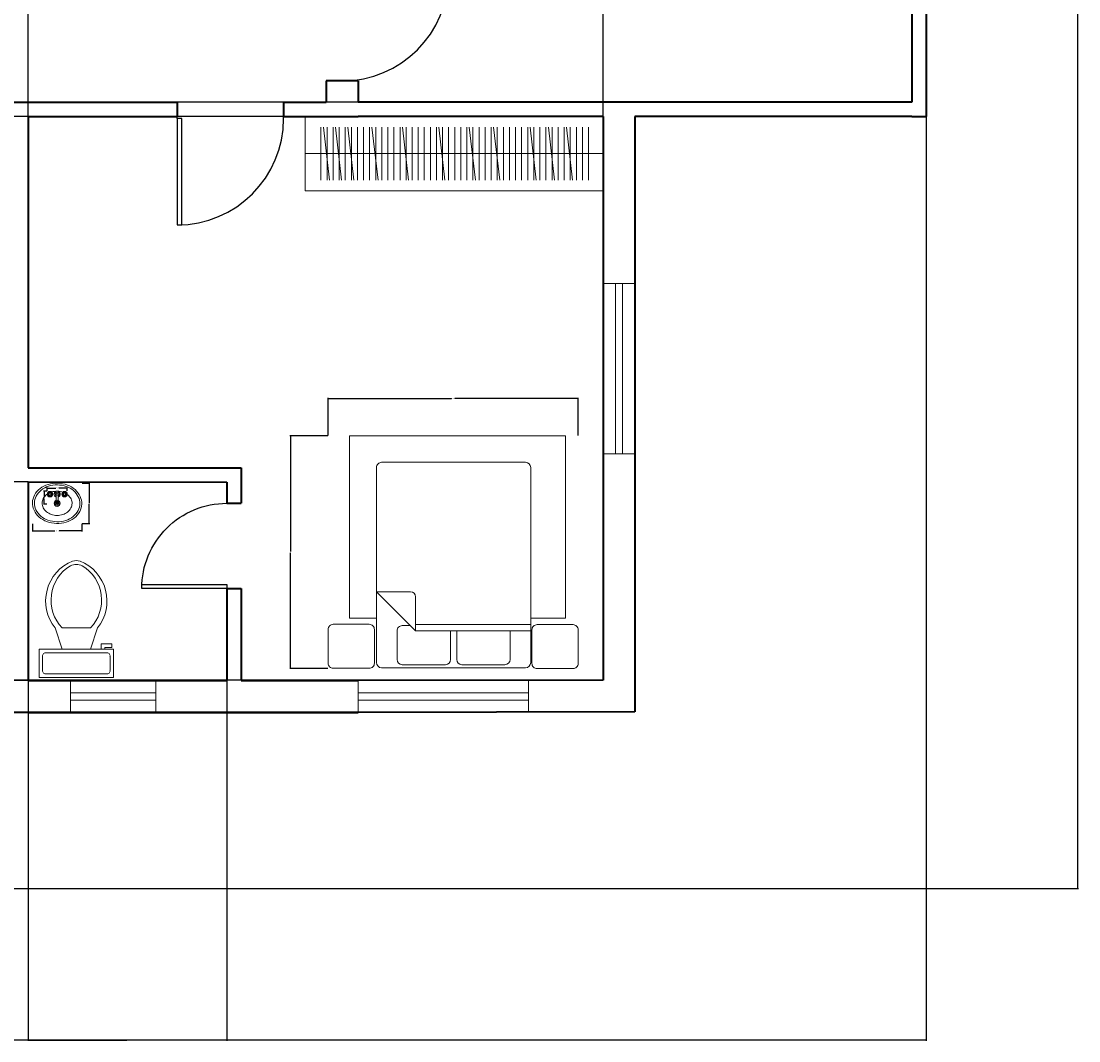
# Model space of a CAD drawing. Units: inches. Extents: x 2024 to 2965, y 1692 to 2308.
# Tile 5 of 8: x 2667 to 2965, y 1692 to 1980. Entities that reach past the tile are written whole.
import ezdxf

# ---------------------------------------------------------------- set-up
doc = ezdxf.new("R2010")
doc.units = ezdxf.units.IN
for name, color, linetype, lineweight in [('A-ANNO-DIMS', 2, 'Continuous', 18), ('A-DOOR', 3, 'Continuous', 25), ('A-FLOR-CASE', 33, 'Continuous', 20), ('A-FLOR-CASE-PATT', 252, 'Continuous', 13), ('A-FLOR-FIXT', 9, 'Continuous', 18), ('A-FURN', 8, 'Continuous', 18), ('A-GLAZ', 4, 'Continuous', 18), ('A-WALL', 7, 'Continuous', 35)]:
    doc.layers.add(name, color=color, linetype=linetype, lineweight=lineweight)
doc.styles.get("Standard").update_dxf_attribs({"font": 'arial.ttf'})
doc.dimstyles.get("Standard").update_dxf_attribs({"dimtxt": 0.18, "dimasz": 0.18, "dimexe": 0.18, "dimexo": 0.0625, "dimgap": 0.09, "dimtad": 0, "dimtih": 1, "dimtoh": 1, "dimdec": 4, "dimzin": 0, "dimdsep": 46, "dimtxsty": 'Standard', "dimcen": 0.09, "dimadec": 0, "dimazin": 0, "dimtfac": 1, "dimtdec": 4, "dimtofl": 0, "dimtmove": 0, "dimatfit": 3, "dimfxl": 1, "dimtolj": 1, "dimtzin": 0, "dimarcsym": 0})

# ---------------------------------------------------------------- blocks, each defined once
blk = doc.blocks.new('*U6')
for p, q in [((0, 0), (0, 6)), ((40, 0), (40, 6))]:
    blk.add_line(p, q)
blk.add_lwpolyline([(0, 0), (0, -40), (1.75, -40), (1.75, 0)], close=True)
blk.add_arc((0, 0), 40, 270, 0)
blk = doc.blocks.new('*U7')
for p, q in [((0, 0), (0, -6)), ((40, 0), (40, -6))]:
    blk.add_line(p, q)
blk.add_lwpolyline([(0, 0), (0, 40), (1.75, 40), (1.75, 0)], close=True)
blk.add_arc((0, 0), 40, 0, 90)
blk = doc.blocks.new('Toilet - top')
for p, q in [((9.5, -6), (9.5, -2)), ((-10, -8.5), (-8, -8.5)), ((-10, -9.5), (-10, -8.5)), ((-8, -8.5), (-8, -8)), ((-7, -8), (-7, -9.5)), ((-4, -8), (-6, -14)), ((4, -8), (6, -14)), ((-7, -9.5), (-10, -9.5)), ((4, -14), (-4, -14))]:
    blk.add_line(p, q)
blk.add_lwpolyline([(10.5, -8), (10.5, 0), (-10.5, 0), (-10.5, -8)], close=True)
for points in [[(-9.5, -2), (-9.5, -6)], [(8.5, -1), (-8.5, -1)], [(-8.5, -7), (8.5, -7)]]:
    blk.add_lwpolyline(points)
for centre, radius, start, end in [((-8.62, -1.88), 0.884, 81.8699, 188.1301), ((8.62, -1.88), 0.884, 351.8699, 98.1301), ((-8.62, -6.12), 0.884, 171.8699, 278.1301), ((8.62, -6.12), 0.884, 261.8699, 8.1301), ((3.52, -21.58), 12.17, 141.4691, 247.9714), ((4.2, -21.82), 11.33, 136.3677, 238.9468), ((-3.52, -21.58), 12.17, 292.0284, 38.5307), ((-4.2, -21.82), 11.33, 301.053, 43.6321), ((0, -27.88), 4, 245.7318, 294.2682), ((0, -29), 4, 254.8605, 285.1395)]:
    blk.add_arc(centre, radius, start, end)
blk = doc.blocks.new('Sink - Oval top')
for p, q in [((-1, 0), (1, 0)), ((0, 1), (0, -1))]:
    blk.add_line(p, q)
for points in [[(-12.23, 0.39, 0.117634), (-11.46, -3.36, 0.104469), (-8.88, -6.8, 0.090016), (-5.08, -9.07, 0.08192), (-0.32, -10.02, 0.08192), (4.49, -9.38, 0.090016), (8.42, -7.36, 0.104469), (11.22, -4.09, 0.117634), (12.23, -0.39, 0.117634), (11.46, 3.36, 0.104469), (8.88, 6.8, 0.090016), (5.08, 9.07, 0.08192), (0.32, 10.02, 0.08192), (-4.49, 9.38, 0.090016), (-8.42, 7.36, 0.104469), (-11.22, 4.09, 0.117634)], [(-11.29, 0.16, 0.118622), (-10.52, -3.25, 0.104678), (-8.07, -6.36, 0.089562), (-4.54, -8.37, 0.081185), (-0.13, -9.15, 0.081185), (4.3, -8.49, 0.089562), (7.89, -6.58, 0.104678), (10.42, -3.55, 0.118622), (11.29, -0.16, 0.118622), (10.52, 3.25, 0.104678), (8.07, 6.36, 0.089562), (4.54, 8.37, 0.081185), (0.13, 9.15, 0.081185), (-4.3, 8.49, 0.089562), (-7.89, 6.58, 0.104678), (-10.42, 3.55, 0.118622)], [(-7.42, 0.08, 0.118283), (-6.91, -2.17, 0.104607), (-5.29, -4.21, 0.089718), (-2.97, -5.53, 0.081436), (-0.07, -6.04, 0.081436), (2.84, -5.59, 0.089718), (5.2, -4.33, 0.104607), (6.86, -2.32, 0.118283), (7.42, -0.08, 0.118283), (6.91, 2.17, 0.104607), (5.29, 4.21, 0.089718), (2.97, 5.53, 0.081436), (0.07, 6.04, 0.081436), (-2.84, 5.59, 0.089718), (-5.2, 4.33, 0.104607), (-6.86, 2.32, 0.118283)]]:
    blk.add_lwpolyline(points, format="xyb", close=True)
for radius in [1.5, 1]:
    blk.add_circle((0, 0), radius)
blk = doc.blocks.new('Faucet - Bathroom top')
for p, q in [((-4.107, 0.125), (-4.375, 0.125)), ((-3.75, 0.4788), (-3.75, 0.75)), ((-3.5, 0.482), (-3.5, 0.75)), ((-3.1461, 0.125), (-2.875, 0.125)), ((3.143, 0.125), (2.875, 0.125)), ((3.5, 0.4788), (3.5, 0.75)), ((3.75, 0.482), (3.75, 0.75)), ((4.1039, 0.125), (4.375, 0.125)), ((-4.1039, -0.125), (-4.375, -0.125)), ((-3.75, -0.4821), (-3.75, -0.75)), ((-3.5, -0.4789), (-3.5, -0.75)), ((-3.143, -0.125), (-2.875, -0.125)), ((-0.5, -0.8639), (-0.5, -4.5)), ((0.5, -4.5), (0.5, -0.8631)), ((3.1461, -0.125), (2.875, -0.125)), ((3.5, -0.4821), (3.5, -0.75)), ((3.75, -0.4789), (3.75, -0.75)), ((4.107, -0.125), (4.375, -0.125))]:
    blk.add_line(p, q)
for centre, radius in [((-3.625, 0), 1.375), ((-4.625, 0), 0.2795), ((-3.625, 0), 0.5), ((-3.625, 1), 0.2795), ((-2.625, 0), 0.2795), ((0, 0), 0.5), ((3.625, 0), 1.375), ((2.625, 0), 0.2795), ((3.625, 0), 0.5), ((3.625, 1), 0.2795), ((4.625, 0), 0.2795), ((-3.625, -1), 0.2795), ((3.625, -1), 0.2795)]:
    blk.add_circle(centre, radius)
for centre, radius, start, end in [((-3.625, 0), 1, 105.2407, 164.2093), ((-3.625, 0), 1, 16.44125, 74.07887), ((0, 0), 1.5, 289.6514, 250.3603), ((0, 0), 1, 300.3431, 239.7554), ((3.625, 0), 1, 106.12, 164.0884), ((3.625, 0), 1, 16.23422, 73.90469), ((-3.625, 0), 1, 196.2342, 253.9047), ((-3.625, 0), 1, 286.12, 344.0884), ((0, -4.5), 0.5, 180, 0), ((3.625, 0), 1, 196.4413, 254.0789), ((3.625, 0), 1, 285.2407, 344.2093)]:
    blk.add_arc(centre, radius, start, end)
blk = doc.blocks.new('Bed - Queen')
for p, q in [((2, 0), (58, 0)), ((0, -78), (0, -2)), ((8, -14.4), (8, -3.2)), ((10, -1.2), (26.8, -1.2)), ((28.8, -3.2), (28.8, -14.4)), ((31.2, -14.4), (31.2, -3.2)), ((33.2, -1.2), (50, -1.2)), ((52, -3.2), (52, -14.4)), ((60, -2), (60, -78)), ((0, -14.4), (44.8, -14.4)), ((60, -29.6), (44.8, -14.4)), ((44.8, -14.4), (44.8, -27.6)), ((50, -16.4), (46.8, -16.4)), ((44.8, -16.8), (0, -16.8)), ((46.8, -29.6), (60, -29.6)), ((58, -80), (2, -80))]:
    blk.add_line(p, q)
for points in [[(-16.47, 0.34), (-2.47, 0.34, -0.414214), (-0.47, -1.66), (-0.47, -14.8, -0.414214), (-2.47, -16.8), (-16.47, -16.8, -0.414214), (-18.47, -14.8), (-18.47, -1.66, -0.414214)], [(62.82, 0.21), (76.82, 0.21, -0.414214), (78.82, -1.79), (78.82, -14.93, -0.414214), (76.82, -16.93), (62.82, -16.93, -0.414214), (60.82, -14.93), (60.82, -1.79, -0.414214)]]:
    blk.add_lwpolyline(points, format="xyb", close=True)
blk.add_lwpolyline([(0, -19.29), (-13.55, -19.29), (-13.55, -90.28), (70.45, -90.28), (70.45, -19.29), (60, -19.29)])
for centre, start, end in [((2, -2), 90, 180), ((58, -2), 0, 90), ((10, -3.2), 90, 180), ((26.8, -3.2), 0, 90), ((33.2, -3.2), 90, 180), ((50, -3.2), 0, 90), ((50, -14.4), 270, 0), ((46.8, -27.6), 180, 270), ((2, -78), 180, 270), ((58, -78), 270, 0)]:
    blk.add_arc(centre, 2, start, end)
blk = doc.blocks.new('WIN-24-D9')
for p, q in [((0, 5.5), (24, 5.5)), ((0, 3.5), (24, 3.5))]:
    blk.add_line(p, q)
for points in [[(0, 0), (0, 9)], [(24, 9), (24, 0)]]:
    blk.add_lwpolyline(points)
blk = doc.blocks.new('WIN-48-D9')
for p, q in [((0, 5.5), (48, 5.5)), ((0, 3.5), (48, 3.5))]:
    blk.add_line(p, q)
for points in [[(0, 0), (0, 9)], [(48, 9), (48, 0)]]:
    blk.add_lwpolyline(points)
blk = doc.blocks.new('*D47')
at = {"layer": 'A-ANNO-DIMS', "color": 0, "lineweight": -2, "transparency": 16777216}
for p, q in [((2753.45, 1862.85), (2753.45, 1873.54)), ((2753.63, 1873.36), (2788.19, 1873.36)), ((2823.77, 1873.36), (2789.21, 1873.36)), ((2823.95, 1862.85), (2823.95, 1873.54))]:
    blk.add_line(p, q, dxfattribs=at)
at = {"layer": 'A-ANNO-DIMS', "color": 0, "transparency": 16777216}
for points in [[(2753.63, 1873.39), (2753.63, 1873.33), (2753.45, 1873.36)], [(2823.77, 1873.39), (2823.77, 1873.33), (2823.95, 1873.36)]]:
    blk.add_solid(points, dxfattribs=at)
at = {"layer": 'Defpoints', "color": 0, "transparency": 16777216}
for p in [(2753.45, 1873.36), (2753.45, 1862.79), (2823.95, 1862.79)]:
    blk.add_point(p, dxfattribs=at)
at = {"layer": 'A-ANNO-DIMS', "color": 0, "transparency": 16777216, "insert": (2788.7, 1873.36), "char_height": 0.18, "attachment_point": 5}
blk.add_mtext('\\A1;BED 70', dxfattribs=at)
blk = doc.blocks.new('*D48')
at = {"layer": 'A-ANNO-DIMS', "color": 0, "lineweight": -2, "transparency": 16777216}
for p, q in [((2753.39, 1862.79), (2742.7, 1862.79)), ((2742.88, 1862.61), (2742.88, 1830.14)), ((2742.88, 1797.31), (2742.88, 1829.78)), ((2753.39, 1797.13), (2742.7, 1797.13))]:
    blk.add_line(p, q, dxfattribs=at)
at = {"layer": 'A-ANNO-DIMS', "color": 0, "transparency": 16777216}
for points in [[(2742.85, 1862.61), (2742.91, 1862.61), (2742.88, 1862.79)], [(2742.85, 1797.31), (2742.91, 1797.31), (2742.88, 1797.13)]]:
    blk.add_solid(points, dxfattribs=at)
at = {"layer": 'Defpoints', "color": 0, "transparency": 16777216}
for p in [(2753.45, 1862.79), (2742.88, 1797.13), (2753.45, 1797.13)]:
    blk.add_point(p, dxfattribs=at)
at = {"layer": 'A-ANNO-DIMS', "color": 0, "transparency": 16777216, "insert": (2742.88, 1829.96), "char_height": 0.18, "attachment_point": 5}
blk.add_mtext('\\A1;66', dxfattribs=at)
blk = doc.blocks.new('*D63')
at = {"layer": 'A-ANNO-DIMS', "color": 0, "lineweight": -2, "transparency": 16777216}
for p, q in [((2670.07, 1837.99), (2670.07, 1835.78)), ((2684.02, 1837.99), (2684.02, 1835.78)), ((2670.25, 1835.96), (2676.42, 1835.96)), ((2683.84, 1835.96), (2677.67, 1835.96))]:
    blk.add_line(p, q, dxfattribs=at)
at = {"layer": 'A-ANNO-DIMS', "color": 0, "transparency": 16777216}
for points in [[(2670.25, 1835.99), (2670.25, 1835.93), (2670.07, 1835.96)], [(2683.84, 1835.99), (2683.84, 1835.93), (2684.02, 1835.96)]]:
    blk.add_solid(points, dxfattribs=at)
at = {"layer": 'Defpoints', "color": 0, "transparency": 16777216}
for p in [(2670.07, 1838.05), (2684.02, 1838.05), (2684.02, 1835.96)]:
    blk.add_point(p, dxfattribs=at)
at = {"layer": 'A-ANNO-DIMS', "color": 0, "transparency": 16777216, "insert": (2677.05, 1835.96), "char_height": 0.18, "attachment_point": 5}
blk.add_mtext('\\A1;BASIN 14', dxfattribs=at)
blk = doc.blocks.new('*D64')
at = {"layer": 'A-ANNO-DIMS', "color": 0, "lineweight": -2, "transparency": 16777216}
for p, q in [((2684.08, 1849.49), (2686.29, 1849.49)), ((2686.11, 1849.31), (2686.11, 1843.95)), ((2686.11, 1838.23), (2686.11, 1843.59)), ((2684.08, 1838.05), (2686.29, 1838.05))]:
    blk.add_line(p, q, dxfattribs=at)
at = {"layer": 'A-ANNO-DIMS', "color": 0, "transparency": 16777216}
for points in [[(2686.08, 1849.31), (2686.14, 1849.31), (2686.11, 1849.49)], [(2686.08, 1838.23), (2686.14, 1838.23), (2686.11, 1838.05)]]:
    blk.add_solid(points, dxfattribs=at)
at = {"layer": 'Defpoints', "color": 0, "transparency": 16777216}
for p in [(2684.02, 1849.49), (2686.11, 1849.49), (2684.02, 1838.05)]:
    blk.add_point(p, dxfattribs=at)
at = {"layer": 'A-ANNO-DIMS', "color": 0, "transparency": 16777216, "insert": (2686.11, 1843.77), "char_height": 0.18, "attachment_point": 5}
blk.add_mtext('\\A1;11', dxfattribs=at)
blk = doc.blocks.new('*D69')
at = {"layer": 'A-ANNO-DIMS', "color": 0, "lineweight": -2, "transparency": 16777216}
for p, q in [((2674.24, 1847.26), (2674.24, 1848.23)), ((2674.42, 1848.05), (2676.65, 1848.05)), ((2679.74, 1848.05), (2677.51, 1848.05)), ((2679.92, 1847.26), (2679.92, 1848.23))]:
    blk.add_line(p, q, dxfattribs=at)
at = {"layer": 'A-ANNO-DIMS', "color": 0, "transparency": 16777216}
for points in [[(2674.42, 1848.08), (2674.42, 1848.02), (2674.24, 1848.05)], [(2679.74, 1848.08), (2679.74, 1848.02), (2679.92, 1848.05)]]:
    blk.add_solid(points, dxfattribs=at)
at = {"layer": 'Defpoints', "color": 0, "transparency": 16777216}
for p in [(2674.24, 1847.2), (2679.92, 1848.05), (2679.92, 1847.2)]:
    blk.add_point(p, dxfattribs=at)
at = {"layer": 'A-ANNO-DIMS', "color": 0, "transparency": 16777216, "insert": (2677.08, 1848.05), "char_height": 0.18, "attachment_point": 5}
blk.add_mtext('\\A1;TAP 6', dxfattribs=at)
blk = doc.blocks.new('*D70')
at = {"layer": 'A-ANNO-DIMS', "color": 0, "lineweight": -2, "transparency": 16777216}
for p, q in [((2674.18, 1847.2), (2673.21, 1847.2)), ((2673.39, 1847.02), (2673.39, 1845.53)), ((2674.18, 1843.5), (2673.21, 1843.5)), ((2673.39, 1843.68), (2673.39, 1845.17))]:
    blk.add_line(p, q, dxfattribs=at)
at = {"layer": 'A-ANNO-DIMS', "color": 0, "transparency": 16777216}
for points in [[(2673.36, 1847.02), (2673.42, 1847.02), (2673.39, 1847.2)], [(2673.36, 1843.68), (2673.42, 1843.68), (2673.39, 1843.5)]]:
    blk.add_solid(points, dxfattribs=at)
at = {"layer": 'Defpoints', "color": 0, "transparency": 16777216}
for p in [(2673.39, 1847.2), (2674.24, 1847.2), (2674.24, 1843.5)]:
    blk.add_point(p, dxfattribs=at)
at = {"layer": 'A-ANNO-DIMS', "color": 0, "transparency": 16777216, "insert": (2673.39, 1845.35), "char_height": 0.18, "attachment_point": 5}
blk.add_mtext('\\A1;4', dxfattribs=at)
blk = doc.blocks.new('*D75')
at = {"layer": 'A-ANNO-DIMS', "color": 0, "lineweight": -2, "transparency": 16777216}
for p, q in [((2922.02, 1952.85), (2922.02, 1692.14)), ((2067.46, 1932.29), (2067.46, 1692.14)), ((2067.64, 1692.32), (2494.35, 1692.32)), ((2921.84, 1692.32), (2495.13, 1692.32))]:
    blk.add_line(p, q, dxfattribs=at)
at = {"layer": 'A-ANNO-DIMS', "color": 0, "transparency": 16777216}
for points in [[(2067.64, 1692.35), (2067.64, 1692.29), (2067.46, 1692.32)], [(2921.84, 1692.35), (2921.84, 1692.29), (2922.02, 1692.32)]]:
    blk.add_solid(points, dxfattribs=at)
at = {"layer": 'Defpoints', "color": 0, "transparency": 16777216}
for p in [(2922.02, 1952.91), (2067.46, 1932.35), (2922.02, 1692.32)]:
    blk.add_point(p, dxfattribs=at)
at = {"layer": 'A-ANNO-DIMS', "color": 0, "transparency": 16777216, "insert": (2494.74, 1692.32), "char_height": 0.18, "attachment_point": 5}
blk.add_mtext('\\A1;854.6', dxfattribs=at)
blk = doc.blocks.new('*D76')
at = {"layer": 'A-ANNO-DIMS', "color": 0, "lineweight": -2, "transparency": 16777216}
for p, q in [((2718.97, 2264.77), (2964.97, 2264.77)), ((2964.79, 2264.59), (2964.79, 2000.12)), ((2964.79, 1735.28), (2964.79, 1999.75)), ((2515.28, 1735.1), (2964.97, 1735.1))]:
    blk.add_line(p, q, dxfattribs=at)
at = {"layer": 'A-ANNO-DIMS', "color": 0, "transparency": 16777216}
for points in [[(2964.76, 2264.59), (2964.82, 2264.59), (2964.79, 2264.77)], [(2964.76, 1735.28), (2964.82, 1735.28), (2964.79, 1735.1)]]:
    blk.add_solid(points, dxfattribs=at)
at = {"layer": 'Defpoints', "color": 0, "transparency": 16777216}
for p in [(2718.91, 2264.77), (2515.22, 1735.1), (2964.79, 1735.1)]:
    blk.add_point(p, dxfattribs=at)
at = {"layer": 'A-ANNO-DIMS', "color": 0, "transparency": 16777216, "insert": (2964.79, 1999.94), "char_height": 0.18, "attachment_point": 5}
blk.add_mtext('\\A1;529.7', dxfattribs=at)
blk = doc.blocks.new('*D99')
at = {"layer": 'A-ANNO-DIMS', "color": 0, "lineweight": -2, "transparency": 16777216}
for p, q in [((2668.91, 1952.85), (2668.91, 2307.73)), ((2669.09, 2307.55), (2749.48, 2307.55)), ((2830.78, 2307.55), (2750.39, 2307.55)), ((2830.96, 1952.97), (2830.96, 2307.73))]:
    blk.add_line(p, q, dxfattribs=at)
at = {"layer": 'A-ANNO-DIMS', "color": 0, "transparency": 16777216}
for points in [[(2669.09, 2307.58), (2669.09, 2307.52), (2668.91, 2307.55)], [(2830.78, 2307.58), (2830.78, 2307.52), (2830.96, 2307.55)]]:
    blk.add_solid(points, dxfattribs=at)
at = {"layer": 'Defpoints', "color": 0, "transparency": 16777216}
for p in [(2830.96, 2307.55), (2668.91, 1952.79), (2830.96, 1952.91)]:
    blk.add_point(p, dxfattribs=at)
at = {"layer": 'A-ANNO-DIMS', "color": 0, "transparency": 16777216, "insert": (2749.93, 2307.55), "char_height": 0.18, "attachment_point": 5}
blk.add_mtext('\\A1;162.06', dxfattribs=at)
blk = doc.blocks.new('*D101')
at = {"layer": 'A-ANNO-DIMS', "color": 0, "lineweight": -2, "transparency": 16777216}
for p, q in [((2917.96, 2113.77), (2024.5, 2113.77)), ((2024.68, 2113.59), (2024.68, 2035.52)), ((2024.68, 1957.09), (2024.68, 2035.16)), ((2917.96, 1956.91), (2024.5, 1956.91))]:
    blk.add_line(p, q, dxfattribs=at)
at = {"layer": 'A-ANNO-DIMS', "color": 0, "transparency": 16777216}
for points in [[(2024.65, 2113.59), (2024.71, 2113.59), (2024.68, 2113.77)], [(2024.65, 1957.09), (2024.71, 1957.09), (2024.68, 1956.91)]]:
    blk.add_solid(points, dxfattribs=at)
at = {"layer": 'Defpoints', "color": 0, "transparency": 16777216}
for p in [(2024.68, 2113.77), (2918.02, 2113.77), (2918.02, 1956.91)]:
    blk.add_point(p, dxfattribs=at)
at = {"layer": 'A-ANNO-DIMS', "color": 0, "transparency": 16777216, "insert": (2024.68, 2035.34), "char_height": 0.18, "attachment_point": 5}
blk.add_mtext('\\A1;156.87', dxfattribs=at)
blk = doc.blocks.new('*D102')
at = {"layer": 'A-ANNO-DIMS', "color": 0, "lineweight": -2, "transparency": 16777216}
for p, q in [((2830.9, 1952.91), (2024.5, 1952.91)), ((2024.68, 1952.73), (2024.68, 1873.58)), ((2024.68, 1794.07), (2024.68, 1873.22)), ((2830.9, 1793.89), (2024.5, 1793.89))]:
    blk.add_line(p, q, dxfattribs=at)
at = {"layer": 'A-ANNO-DIMS', "color": 0, "transparency": 16777216}
for points in [[(2024.65, 1952.73), (2024.71, 1952.73), (2024.68, 1952.91)], [(2024.65, 1794.07), (2024.71, 1794.07), (2024.68, 1793.89)]]:
    blk.add_solid(points, dxfattribs=at)
at = {"layer": 'Defpoints', "color": 0, "transparency": 16777216}
for p in [(2830.96, 1952.91), (2024.68, 1793.89), (2830.96, 1793.89)]:
    blk.add_point(p, dxfattribs=at)
at = {"layer": 'A-ANNO-DIMS', "color": 0, "transparency": 16777216, "insert": (2024.68, 1873.4), "char_height": 0.18, "attachment_point": 5}
blk.add_mtext('\\A1;159', dxfattribs=at)
blk = doc.blocks.new('*D110')
at = {"layer": 'A-ANNO-DIMS', "color": 0, "lineweight": -2, "transparency": 16777216}
for p, q in [((2668.91, 1793.71), (2668.91, 1692.14)), ((2724.91, 1793.71), (2724.91, 1692.14)), ((2669.09, 1692.32), (2696.69, 1692.32)), ((2724.73, 1692.32), (2697.12, 1692.32))]:
    blk.add_line(p, q, dxfattribs=at)
at = {"layer": 'A-ANNO-DIMS', "color": 0, "transparency": 16777216}
for points in [[(2669.09, 1692.35), (2669.09, 1692.29), (2668.91, 1692.32)], [(2724.73, 1692.35), (2724.73, 1692.29), (2724.91, 1692.32)]]:
    blk.add_solid(points, dxfattribs=at)
at = {"layer": 'Defpoints', "color": 0, "transparency": 16777216}
for p in [(2668.91, 1793.77), (2724.91, 1793.77), (2724.91, 1692.32)]:
    blk.add_point(p, dxfattribs=at)
at = {"layer": 'A-ANNO-DIMS', "color": 0, "transparency": 16777216, "insert": (2696.91, 1692.32), "char_height": 0.18, "attachment_point": 5}
blk.add_mtext('\\A1;56', dxfattribs=at)
blk = doc.blocks.new('*D111')
at = {"layer": 'A-ANNO-DIMS', "color": 0, "lineweight": -2, "transparency": 16777216}
for p, q in [((2668.84, 1849.79), (2024.5, 1849.79)), ((2024.68, 1849.61), (2024.68, 1821.96)), ((2024.68, 1793.95), (2024.68, 1821.6)), ((2668.84, 1793.77), (2024.5, 1793.77))]:
    blk.add_line(p, q, dxfattribs=at)
at = {"layer": 'A-ANNO-DIMS', "color": 0, "transparency": 16777216}
for points in [[(2024.65, 1849.61), (2024.71, 1849.61), (2024.68, 1849.79)], [(2024.65, 1793.95), (2024.71, 1793.95), (2024.68, 1793.77)]]:
    blk.add_solid(points, dxfattribs=at)
at = {"layer": 'Defpoints', "color": 0, "transparency": 16777216}
for p in [(2024.68, 1849.79), (2668.91, 1849.79), (2668.91, 1793.77)]:
    blk.add_point(p, dxfattribs=at)
at = {"layer": 'A-ANNO-DIMS', "color": 0, "transparency": 16777216, "insert": (2024.68, 1821.78), "char_height": 0.18, "attachment_point": 5}
blk.add_mtext('\\A1;56.01', dxfattribs=at)

msp = doc.modelspace()

# ---------------------------------------------------------------- hatches: boundary and pattern name
at = {"layer": 'A-FLOR-CASE-PATT'}
h = msp.add_hatch(dxfattribs=at)
h.set_pattern_fill('ANSI31', color=256, scale=0.5399325, angle=45, style=0)
h.paths.add_polyline_path([(2750.3912, 1934.9082), (2827.5341, 1934.9082), (2827.5341, 1949.9082), (2750.3912, 1949.9082)])

# ---------------------------------------------------------------- linework, layer by layer
at = {"layer": 'A-FLOR-CASE'}
for p, q in [((2830.9627, 1952.9082), (2746.9627, 1952.9082)), ((2746.9627, 1952.9082), (2746.9627, 1931.9082)), ((2830.9627, 1931.9082), (2830.9627, 1952.9082)), ((2830.9627, 1952.9082), (2830.9627, 1931.9082)), ((2746.9627, 1942.4082), (2830.9627, 1942.4082)), ((2746.9627, 1931.9082), (2830.9627, 1931.9082))]:
    msp.add_line(p, q, dxfattribs=at)
at = {"layer": 'A-FLOR-CASE-PATT'}
for p, q in [((2752.1055, 1949.9082), (2753.8198, 1934.9082)), ((2755.5341, 1949.9082), (2757.2484, 1934.9082)), ((2758.9627, 1949.9082), (2760.6769, 1934.9082)), ((2765.8198, 1949.9082), (2767.5341, 1934.9082)), ((2774.3912, 1949.9082), (2776.1055, 1934.9082)), ((2784.6769, 1949.9082), (2786.3912, 1934.9082)), ((2793.2484, 1949.9082), (2794.9627, 1934.9082)), ((2800.1055, 1949.9082), (2801.8198, 1934.9082)), ((2810.3912, 1949.9082), (2812.1055, 1934.9082)), ((2815.5341, 1949.9082), (2817.2484, 1934.9082)), ((2820.6769, 1949.9082), (2822.3912, 1934.9082))]:
    msp.add_line(p, q, dxfattribs=at)
at = {"layer": 'A-WALL'}
for p, q in [((2922.0192, 2117.7736), (2922.0192, 1952.9082)), ((2918.0192, 2113.7736), (2918.0192, 1956.9082)), ((2761.9061, 1962.9082), (2752.9061, 1962.9082)), ((2752.9061, 1962.9082), (2752.9061, 1956.7881)), ((2668.9061, 1956.7881), (2664.9061, 1956.7881)), ((2710.9061, 1956.7881), (2668.9061, 1956.7881)), ((2710.9061, 1956.7881), (2710.9061, 1952.7881)), ((2752.9061, 1956.7881), (2740.9061, 1956.7881)), ((2740.9061, 1956.7881), (2740.9061, 1952.7881)), ((2918.0192, 1956.9082), (2761.9061, 1956.9082)), ((2668.9061, 1952.7881), (2668.9061, 1853.7881)), ((2710.9061, 1952.7881), (2668.9061, 1952.7881)), ((2761.9061, 1952.7881), (2740.9061, 1952.7881)), ((2830.9627, 1952.9082), (2761.9061, 1952.9082)), ((2830.9627, 1952.9082), (2830.9627, 1793.8927)), ((2918.0192, 1952.9082), (2839.9627, 1952.9082)), ((2839.9627, 1952.9082), (2839.9627, 1784.9082)), ((2918.0192, 1952.9082), (2922.0192, 1952.9082)), ((2668.9061, 1853.7881), (2728.9061, 1853.7787)), ((2728.9061, 1853.7787), (2728.9061, 1843.7794)), ((2668.9061, 1849.7881), (2724.9061, 1849.7794)), ((2668.9061, 1849.7881), (2668.9061, 1793.7736)), ((2724.9061, 1849.7794), (2724.9061, 1843.7794)), ((2724.9061, 1843.7794), (2728.9061, 1843.7794)), ((2724.9061, 1819.7794), (2728.9061, 1819.7794)), ((2724.9061, 1819.7794), (2724.9061, 1793.7736)), ((2728.9061, 1819.7794), (2728.9061, 1793.7736)), ((2668.9075, 1793.7881), (2724.9061, 1793.7794)), ((2728.9061, 1793.7787), (2761.9075, 1793.7736)), ((2830.9627, 1793.8927), (2761.8906, 1793.7736)), ((2668.9061, 1784.7881), (2761.9061, 1784.7736)), ((2839.9627, 1784.9082), (2761.9061, 1784.7736))]:
    msp.add_line(p, q, dxfattribs=at)
for points in [[(2761.9061, 1962.9082), (2761.9061, 1956.9082)], [(2761.9061, 1952.9082), (2761.9061, 1952.7881)], [(2761.9061, 1784.7736), (2664.9061, 1784.7736)]]:
    msp.add_lwpolyline(points, dxfattribs=at)

# ---------------------------------------------------------------- block references
at = {"layer": 'A-DOOR', "rotation": 270}
for name, p, xscale, yscale, zscale in [('*U7', (2757.4061, 1992.9082), 0.75, 0.75, 0.75), ('*U6', (2724.9061, 1819.7794), -0.6, 0.6, 0.6)]:
    msp.add_blockref(name, p, dxfattribs=dict(at, xscale=xscale, yscale=yscale, zscale=zscale))
at = {"layer": 'A-DOOR', "xscale": 0.75, "yscale": 0.75, "zscale": 0.75}
msp.add_blockref('*U6', (2710.9061, 1952.2881), dxfattribs=at)
at = {"layer": 'A-FLOR-FIXT', "xscale": 0.5679565492086411, "yscale": 0.5679565492086411, "zscale": 0.5679565492086411}
for name, p in [('Sink - Oval top', (2677.0454, 1843.7674)), ('Faucet - Bathroom top', (2677.0839, 1846.3441))]:
    msp.add_blockref(name, p, dxfattribs=at)
at = {"layer": 'A-FLOR-FIXT', "rotation": 180}
msp.add_blockref('Toilet - top', (2682.4582, 1794.6252), dxfattribs=at)
at = {"layer": 'A-FURN', "xscale": 0.7245245443840465, "yscale": 0.7245245443840465, "zscale": 0.7245245443840465, "rotation": 180}
msp.add_blockref('Bed - Queen', (2810.5609, 1797.3782), dxfattribs=at)
at = {"layer": 'A-GLAZ', "rotation": 270.000000000001}
msp.add_blockref('WIN-48-D9', (2830.9631, 1905.7282), dxfattribs=at)
at = {"layer": 'A-GLAZ'}
for name, p in [('WIN-24-D9', (2680.8503, 1784.774)), ('WIN-48-D9', (2761.9063, 1784.774))]:
    msp.add_blockref(name, p, dxfattribs=at)

# ---------------------------------------------------------------- dimensions: what is measured, and where the dimension line sits
at = {"layer": 'A-ANNO-DIMS'}
for base, p1, p2, override, picture, middle in [((2830.9627, 2307.5486), (2668.9061, 1952.7881), (2830.9627, 1952.9082), {"dimdec": 2, "dimlfac": 1, "dimrnd": 0, "dimzin": 0, "dimdsep": 46, "dimlunit": 2}, '*D99', (2749.9344, 2307.5486)), ((2922.0192, 1692.3236), (2067.4594, 1932.352), (2922.0192, 1952.9082), {"dimdec": 1, "dimlfac": 1, "dimrnd": 0, "dimzin": 0, "dimdsep": 46, "dimlunit": 2}, '*D75', (2494.7393, 1692.3236)), ((2724.9061, 1692.3236), (2668.9061, 1793.7736), (2724.9061, 1793.7736), {"dimdec": 0, "dimlfac": 1, "dimrnd": 0, "dimzin": 0, "dimdsep": 46, "dimlunit": 2}, '*D110', (2696.9061, 1692.3236))]:
    dim = msp.add_linear_dim(base=base, p1=p1, p2=p2, dimstyle='Standard', override=override, dxfattribs=at)
    dim.commit()
    dim.dimension.update_dxf_attribs({"geometry": picture, "text_midpoint": middle})
for base, p1, p2, angle, override, picture, middle in [((2964.7942, 1735.0986), (2718.9061, 2264.7736), (2515.2195, 1735.0986), 90, {"dimdec": 1, "dimlfac": 1, "dimrnd": 0, "dimzin": 0, "dimdsep": 46, "dimlunit": 2}, '*D76', (2964.7942, 1999.9361)), ((2024.6844, 2113.7736), (2918.0192, 1956.9082), (2918.0192, 2113.7736), 90, {"dimdec": 2, "dimlfac": 1, "dimrnd": 0, "dimzin": 0, "dimdsep": 46, "dimlunit": 2}, '*D101', (2024.6844, 2035.3409)), ((2024.6844, 1793.8927), (2830.9627, 1952.9082), (2830.9627, 1793.8927), 90, {"dimdec": 0, "dimlfac": 1, "dimrnd": 0, "dimzin": 0, "dimdsep": 46, "dimlunit": 2}, '*D102', (2024.6844, 1873.4004)), ((2742.8781, 1797.1314), (2753.4521, 1862.7869), (2753.4521, 1797.1314), 270, {"dimdec": 0, "dimlfac": 1, "dimrnd": 0, "dimzin": 0, "dimdsep": 46, "dimlunit": 2}, '*D48', (2742.8781, 1829.9592)), ((2024.6844, 1849.7881), (2668.9061, 1793.7736), (2668.9061, 1849.7881), 90, {"dimdec": 2, "dimlfac": 1, "dimrnd": 0, "dimzin": 0, "dimdsep": 46, "dimlunit": 2}, '*D111', (2024.6844, 1821.7809)), ((2686.1089, 1849.4857), (2684.0173, 1838.049), (2684.0173, 1849.4857), 90, {"dimdec": 0, "dimlfac": 1, "dimrnd": 0, "dimzin": 0, "dimdsep": 46, "dimlunit": 2}, '*D64', (2686.1089, 1843.7674)), ((2673.3921, 1847.1961), (2674.2441, 1843.5043), (2674.2441, 1847.1961), 90, {"dimdec": 0, "dimlfac": 1, "dimrnd": 0, "dimzin": 0, "dimdsep": 46, "dimlunit": 2}, '*D70', (2673.3921, 1845.3502))]:
    dim = msp.add_linear_dim(base=base, p1=p1, p2=p2, angle=angle, dimstyle='Standard', override=override, dxfattribs=at)
    dim.commit()
    dim.dimension.update_dxf_attribs({"geometry": picture, "text_midpoint": middle})
dim = msp.add_linear_dim(base=(2753.4521, 1873.3609), p1=(2823.9454, 1862.7869), p2=(2753.4521, 1862.7869), angle=180, text='BED <>', dimstyle='Standard', override={"dimdec": 0, "dimlfac": 1, "dimrnd": 0, "dimzin": 0, "dimdsep": 46, "dimlunit": 2}, dxfattribs=at)
dim.commit()
dim.dimension.update_dxf_attribs({"geometry": '*D47', "text_midpoint": (2788.6988, 1873.3609)})
for base, p1, p2, text, picture, middle in [((2679.9236, 1848.048), (2674.2441, 1847.1961), (2679.9236, 1847.1961), 'TAP <>', '*D69', (2677.0839, 1848.048)), ((2684.0173, 1835.9574), (2670.0735, 1838.049), (2684.0173, 1838.049), 'BASIN <>', '*D63', (2677.0454, 1835.9574))]:
    dim = msp.add_linear_dim(base=base, p1=p1, p2=p2, text=text, dimstyle='Standard', override={"dimdec": 0, "dimlfac": 1, "dimrnd": 0, "dimzin": 0, "dimdsep": 46, "dimlunit": 2}, dxfattribs=at)
    dim.commit()
    dim.dimension.update_dxf_attribs({"geometry": picture, "text_midpoint": middle})

doc.saveas('drawing.dxf')
